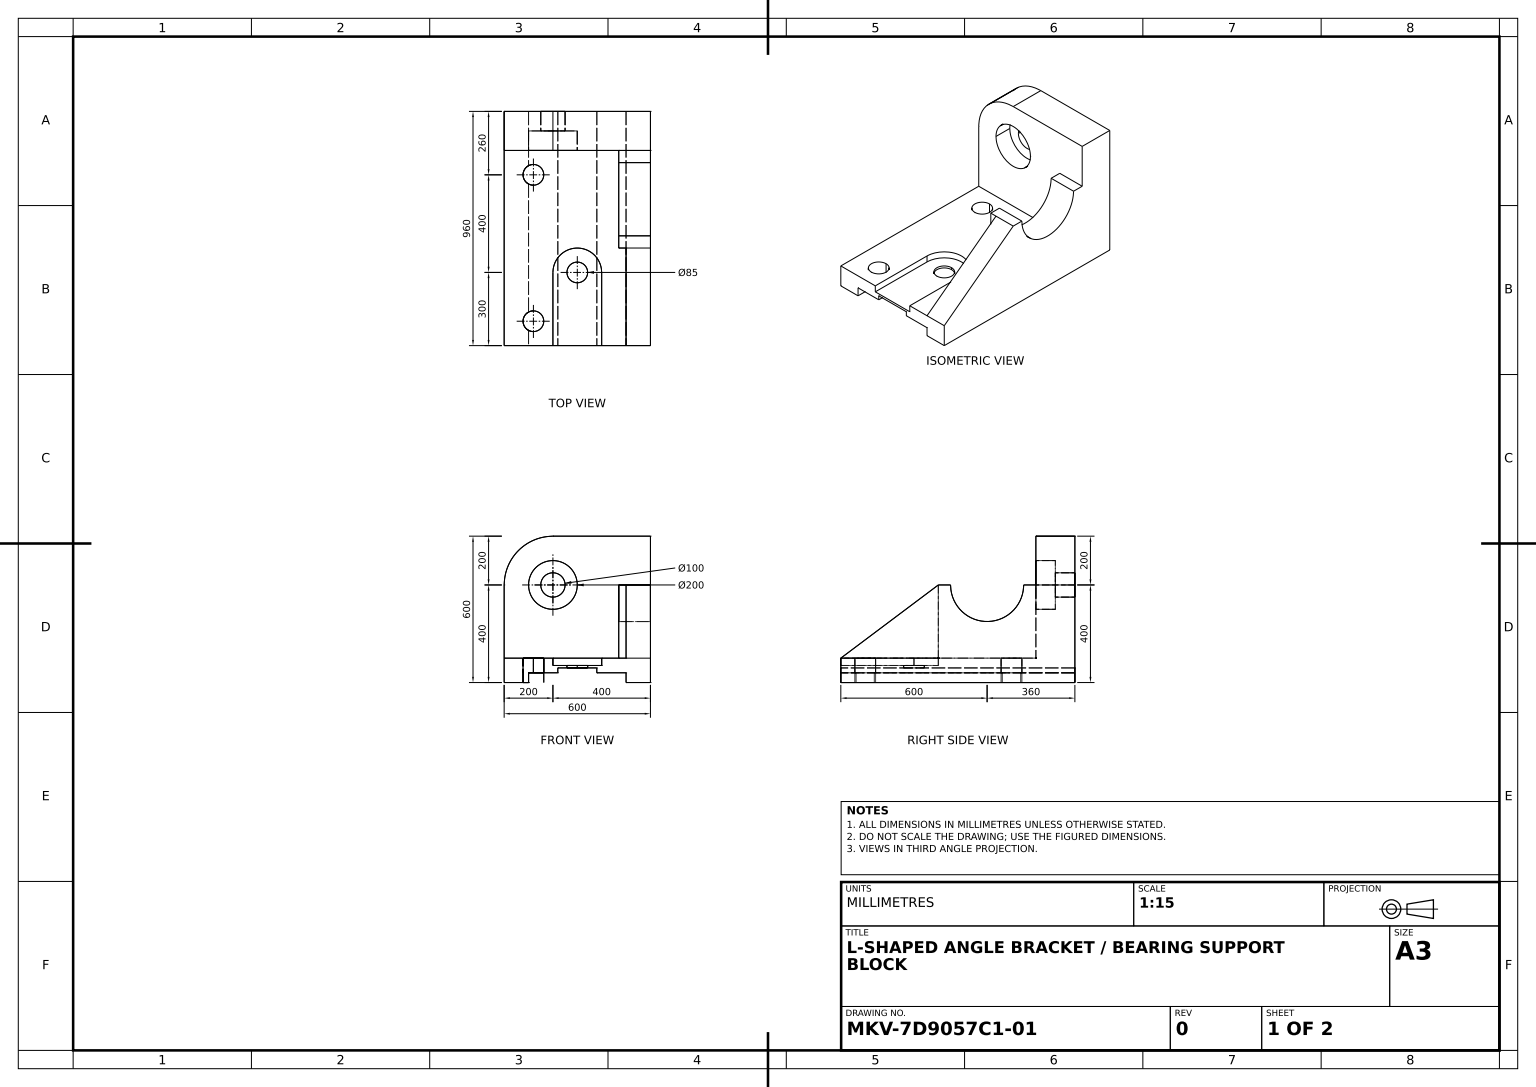
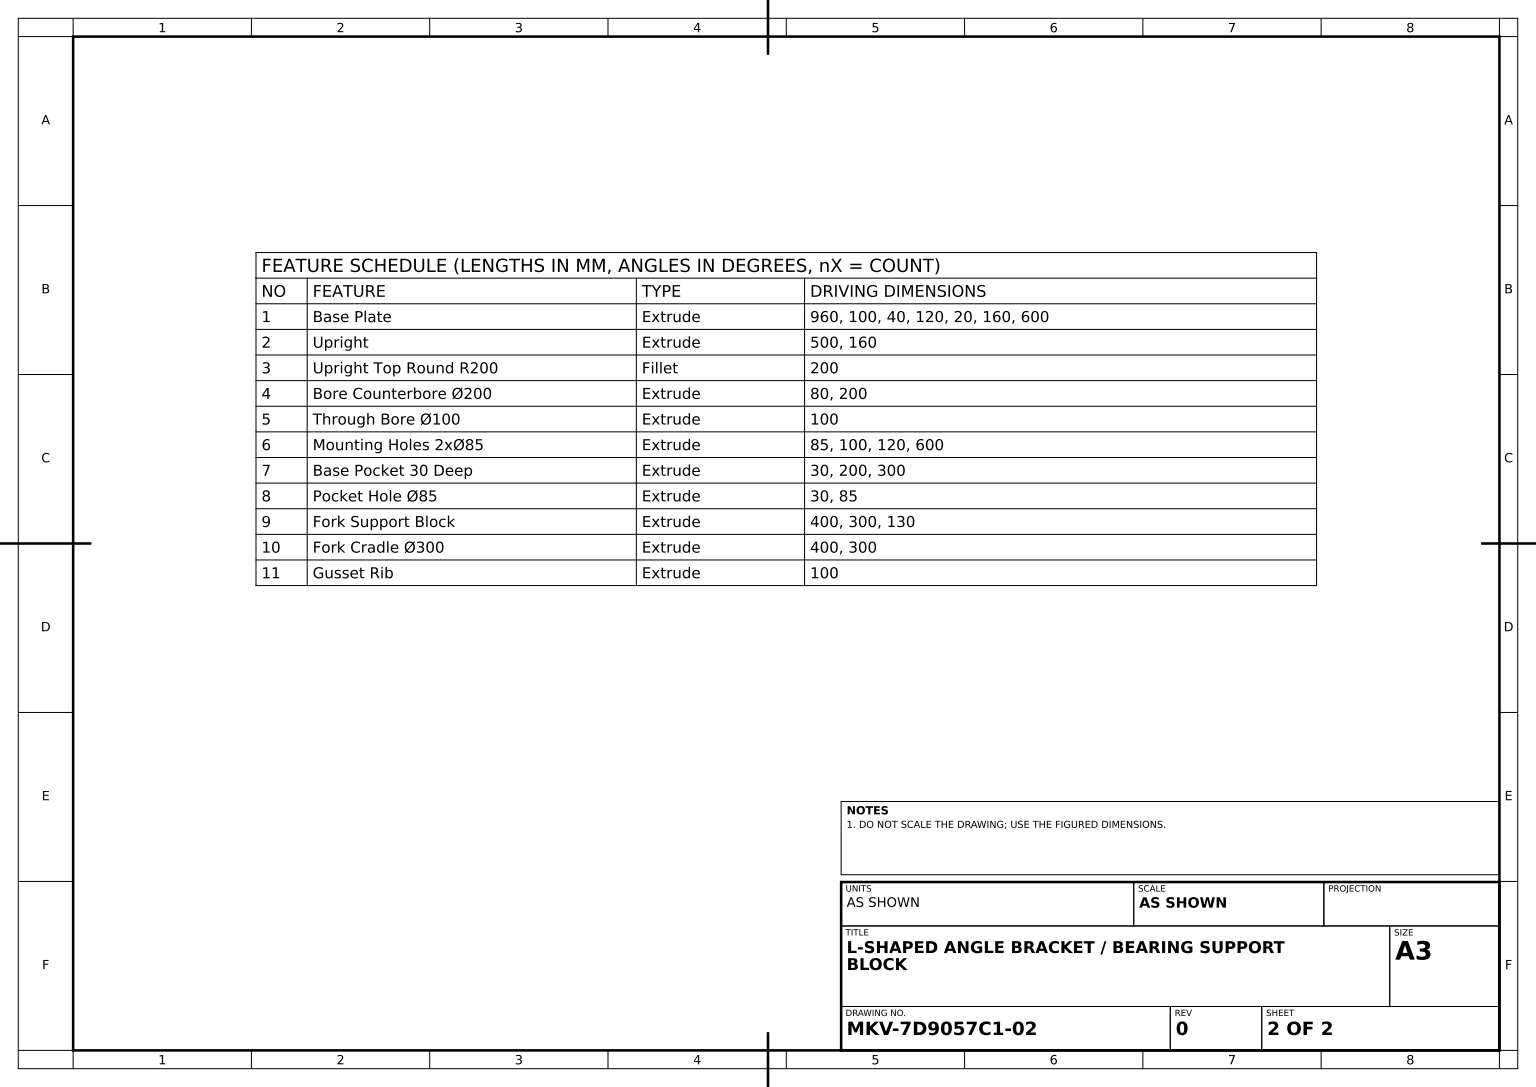
SolidWorks part; units mm, degrees
material "Plain Carbon Steel"
ref_plane "Front Plane" through (0, 0, 0) normal (0, 0, 1) x (1, 0, 0)
ref_plane "Top Plane" through (0, 0, 0) normal (0, 1, 0) x (1, 0, 0)
ref_plane "Right Plane" through (0, 0, 0) normal (1, 0, 0) x (0, 0, -1)
sketch "Base Plate Profile Sketch" plane through (0, 0, 0) normal (0, 0, 1) x (1, 0, 0)
  line L0 (0, 0) -> (100, 0)
  line L1 (100, 0) -> (100, 40)
  line L2 (100, 40) -> (220, 40)
  line L3 (220, 40) -> (220, 60)
  line L4 (220, 60) -> (380, 60)
  line L5 (380, 60) -> (380, 40)
  line L6 (380, 40) -> (500, 40)
  line L7 (500, 40) -> (500, 0)
  line L8 (500, 0) -> (600, 0)
  line L9 (600, 0) -> (600, 100)
  line L10 (600, 100) -> (0, 100)
  line L11 (0, 100) -> (0, 0)
  dimension "D1" = 100
  dimension "D2" = 40
  dimension "D3" = 120
  dimension "D4" = 20
  dimension "D5" = 160
  dimension "D6" = 20
  dimension "D7" = 120
  dimension "D8" = 100
  dimension "D9" = 600
extrude "Base Plate" add sketch "Base Plate Profile Sketch" against normal blind 960
sketch "Upright Sketch" plane through (0, 100, 0) normal (0, 1, 0) x (1, 0, 0)
  line L0 (600, 960) -> (600, 0) construction
  line L1 (0, 960) -> (600, 960)
  line L2 (0, 960) -> (0, 800)
  line L3 (0, 800) -> (600, 800)
  line L4 (600, 960) -> (600, 800)
  dimension "D1" = 160
extrude "Upright" add sketch "Upright Sketch" along normal blind 500
fillet "Upright Top Round R200" radius 200 1 edges at (0, 600, -880)
sketch "Bore Counterbore Sketch" plane through (0, 0, -800) normal (0, 0, 1) x (1, 0, 0)
  circle A0 centre (200, 400) radius 100
  dimension "D1" = 200
extrude "Bore Counterbore Ø200" cut sketch "Bore Counterbore Sketch" against normal blind 80
sketch "Through Bore Sketch" plane through (0, 0, -880) normal (0, 0, 1) x (1, 0, 0)
  circle A0 centre (200, 400) radius 50
  dimension "D1" = 100
extrude "Through Bore Ø100" cut sketch "Through Bore Sketch" against normal through all
sketch "Mounting Holes Sketch" plane through (0, 100, 0) normal (0, 1, 0) x (1, 0, 0)
  line L0 (0, 800) -> (600, 800) construction
  line L1 (0, 800) -> (0, 0) construction
  circle A0 centre (120, 700) radius 42.5
  circle A1 centre (120, 100) radius 42.5
  dimension "D1" = 85
  dimension "85" = 85
  dimension "D3" = 100
  dimension "D4" = 120
  dimension "D5" = 600
  dimension "D6" = 120
extrude "Mounting Holes 2xØ85" cut sketch "Mounting Holes Sketch" against normal through all
sketch "Base Pocket Sketch" plane through (0, 100, 0) normal (0, 1, 0) x (1, 0, 0)
  line L0 (600, 0) -> (0, 0) construction
  line L1 (200, 300) -> (200, 0)
  line L2 (200, 0) -> (400, 0)
  line L3 (400, 0) -> (400, 300)
  arc A0 (400, 300) -> (200, 300) centre (300, 300) ccw
  dimension "D1" = 200
  dimension "D4" = 200
  dimension "D2" = 300
  dimension "D3" = 300
extrude "Base Pocket 30 Deep" cut sketch "Base Pocket Sketch" against normal blind 30
sketch "Pocket Hole Sketch" plane through (0, 70, 0) normal (0, 1, 0) x (1, 0, 0)
  circle A0 centre (300, 300) radius 42.5
  dimension "D1" = 85
extrude "Pocket Hole Ø85" cut sketch "Pocket Hole Sketch" against normal blind 30
sketch "Fork Support Block Sketch" plane through (0, 0, -800) normal (0, 0, 1) x (1, 0, 0)
  line L1 (600, 100) -> (470, 100)
  line L2 (600, 100) -> (600, 400)
  line L3 (600, 400) -> (470, 400)
  line L4 (470, 100) -> (470, 400)
  dimension "D1" = 300
  dimension "D2" = 130
extrude "Fork Support Block" add sketch "Fork Support Block Sketch" along normal blind 400
sketch "Fork Cradle Sketch" plane through (600, 0, 0) normal (1, 0, 0) x (0, 0, -1)
  line L0 (400, 400) -> (800, 400) construction
  circle A0 centre (600, 400) radius 150
  dimension "D1" = 300
extrude "Fork Cradle Ø300" cut sketch "Fork Cradle Sketch" against normal blind 400
sketch "Gusset Rib Sketch" plane through (600, 0, 0) normal (1, 0, 0) x (0, 0, -1)
  line L0 (400, 400) -> (400, 100)
  line L1 (400, 100) -> (0, 100)
  line L2 (0, 100) -> (400, 400)
extrude "Gusset Rib" add sketch "Gusset Rib Sketch" against normal blind 100
